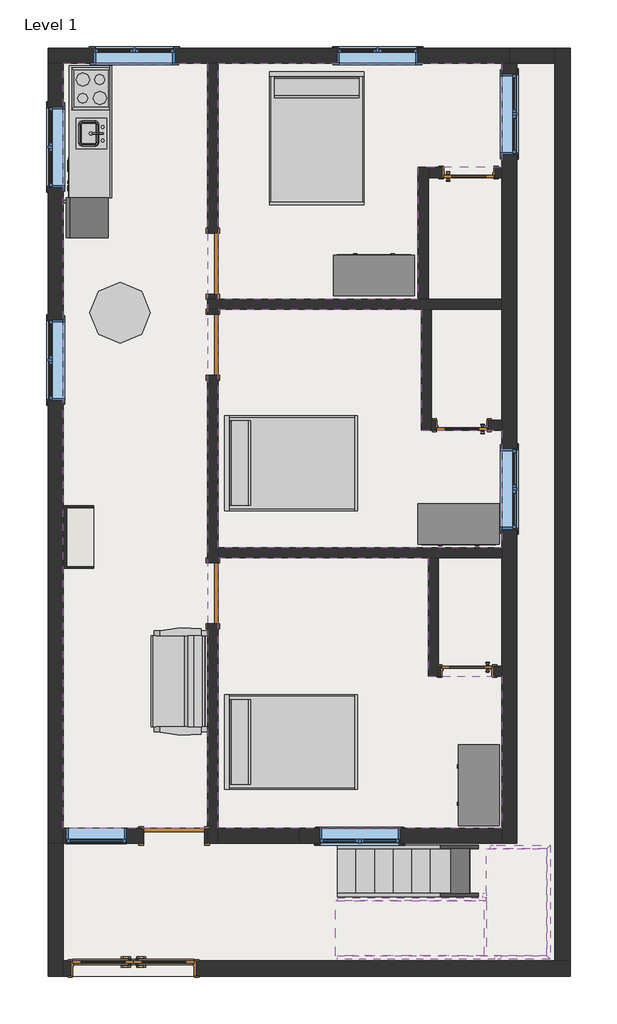
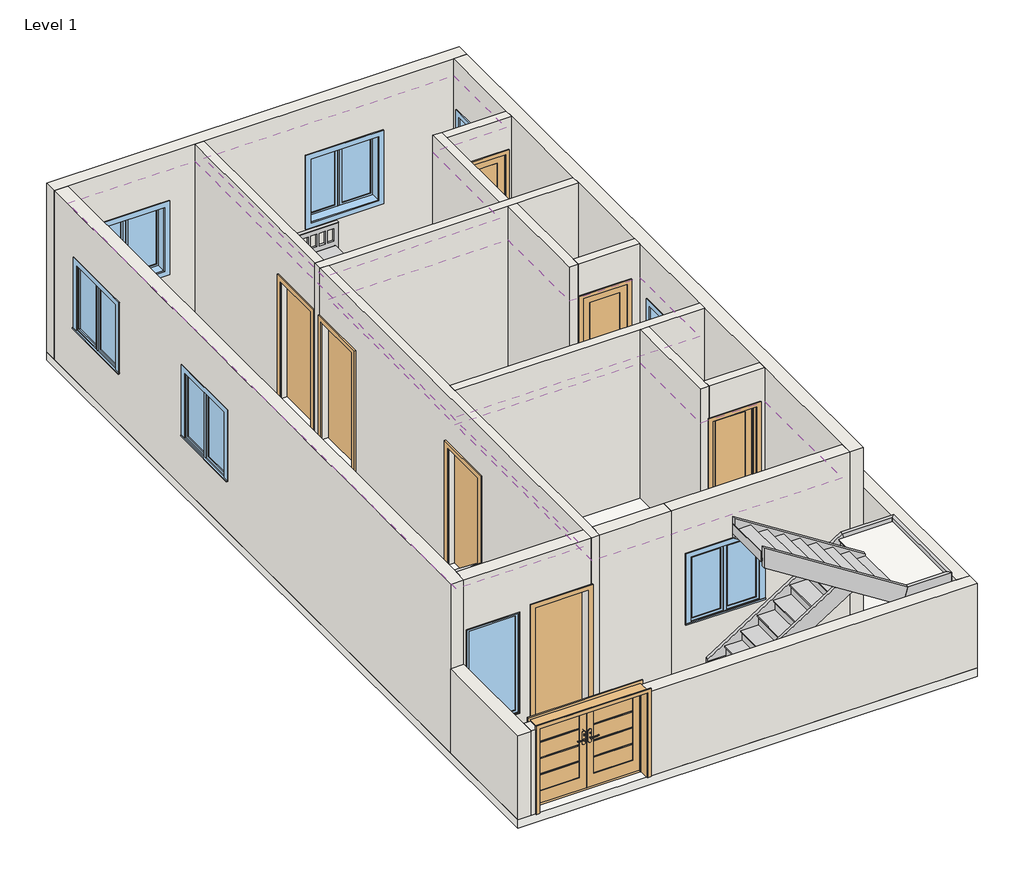
# One storey, incomplete: 21 walls, 9 furniture elements, 8 doors, 8 members, 8 windows, 4 coverings, 4 proxies, 2 slabs, 3 other elements.
# Revit data of these elements (continued)
# Materials (continued)
#   "Glass": class "Glass", colour RGB 0 128 192, transparency 0.75, Description = "Soda Lime Glass", Cost = 0
#   "Aluminum": class "Metal", colour RGB 247 247 247, transparency 0, Description = "Aluminum 6061", Cost = 0
#   "Door - Panel": class "Wood", colour RGB 210 159 95, transparency 0
#   "Door - Frame": colour RGB 118 70 51, transparency 0
#   "Birch": class "Wood", colour RGB 224 178 126, transparency 0, Description = "Betula Alleghaniensis", Cost = 0
#   "Linen, White": class "Textile", colour RGB 247 247 239, transparency 0, Description = "Linen, white", Cost = 0
#   "Laminate - Ivory, Glossy": colour RGB 247 247 239, transparency 0
#   "Laminate, Ivory, Matte": class "Plastic", colour RGB 247 247 239, transparency 0, Description = "Plastic Laminate - Ivory, Matte", Cost = 0
#   "Linen, Beige": class "Textile", colour RGB 249 239 230, transparency 0, Description = "Linen, beige", Cost = 0
#   "Pine": class "Wood", colour RGB 223 192 134, transparency 0, Description = "Pinus Echinata", Cost = 0
#   "Laminate, Linen, Matte": class "Plastic", colour RGB 249 239 230, transparency 0, Description = "Plastic Laminate - Linen, Matte", Cost = 0
#   "FLOOR": class "Generic", colour RGB 144 129 110, transparency 0, Cost = 0
#   "EXT WALL": class "Generic", colour RGB 120 120 120, transparency 0, Cost = 0
#   "Sash": class "Wood", colour RGB 224 178 126, transparency 0
#   "Trim": class "Wood", colour RGB 224 178 126, transparency 0
#   "Counter Top": class "Wood", colour RGB 226 177 128, transparency 0
#   "Default Wall": colour RGB 128 128 128, transparency 0
